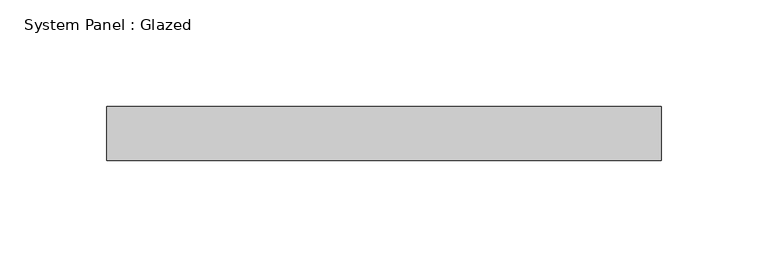
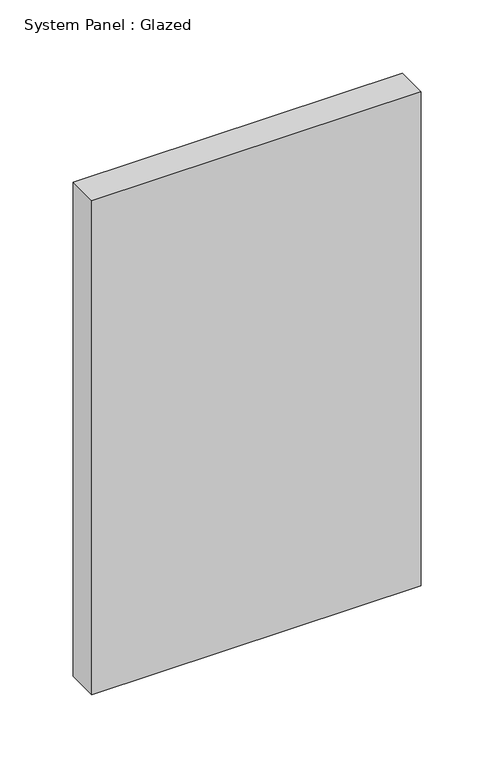
"""IFC4 building model written with IfcOpenShell, lengths in millimetres: plate geometry, System Panel : Glazed."""

from ifc_helpers import new_model, si_unit, origin, origin_with_axes, place, context, project, spatial, polyline, outline, extrude, source, transform, mapped, element, save


def system_panel_glazed_d839e02d(model_context):
    return source(origin(), model_context, "Body", "SweptSolid", [
        extrude(outline(polyline([(130.175, 19.05), (-130.175, 19.05), (-130.175, 44.45), (130.175, 44.45), (130.175, 19.05)])), origin_with_axes(), (0.0, 0.0, 1.0), 412.75),
    ])


if __name__ == "__main__":
    model = new_model("IFC4")
    model_context = context("Model", 3, world=origin())
    ifc_project = project(units=[si_unit("LENGTHUNIT", "METRE", prefix="MILLI")], contexts=[model_context])
    site = spatial("IfcSite", under=ifc_project)
    building = spatial("IfcBuilding", under=site)
    placement = place(None, origin())
    system_panel_glazed_shape = system_panel_glazed_d839e02d(model_context)
    element("IfcPlate", 1, ObjectType="System Panel : Glazed", at=placement, inside=building, context=model_context, shape_type="MappedRepresentation", body=[
        mapped(system_panel_glazed_shape, transform((0.0, 0.0, 0.0), x_axis=(1.0, 0.0, 0.0), y_axis=(0.0, 1.0, 0.0), z_axis=(0.0, 0.0, 1.0))),
    ])
    save(model, "model.ifc")

# Revit data of these elements
# Type "System Panel : Glazed"
#   Construction Type Id = "GSP4R"
#   Analytic Construction = "1/8 in Pilkington single glazing"
#   Visual Light Transmittance = 0.9
#   Solar Heat Gain Coefficient = 0.86
#   Heat Transfer Coefficient (U) = 1.18115 BTU/(h·ft²·°F)
#   Define Thermal Properties by = 1
# Element 1 (IfcPlate, "System Panel : Glazed")
#   Materials on its faces: "Glass"
# Materials
#   "Glass": class "Glass", colour RGB 0 128 192, transparency 0.75, Description = "Soda Lime Glass", Cost = 0
